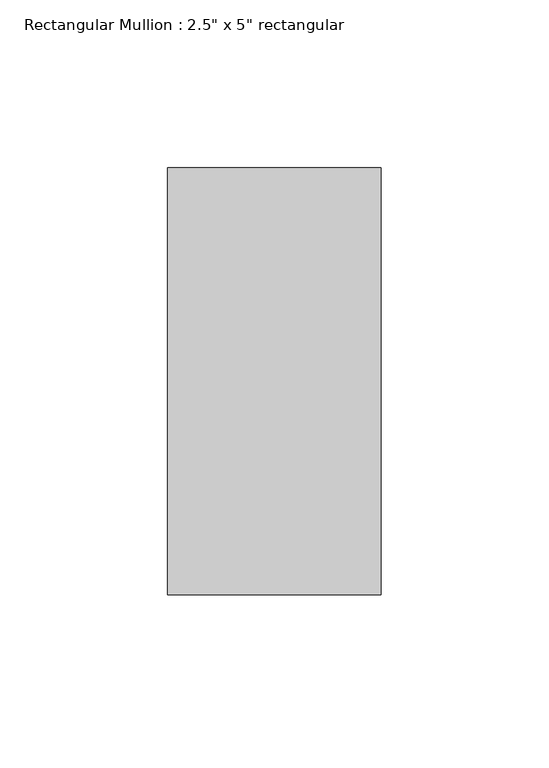
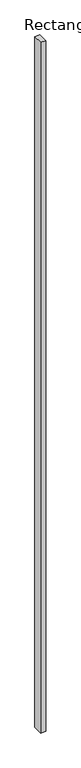
"""IFC4 building model written with IfcOpenShell, lengths in millimetres: member geometry."""

from ifc_helpers import new_model, si_unit, frame, origin, place, context, project, spatial, polyline, outline, extrude, source, transform, mapped, element, save


def member_5f6c94d3(model_context):
    return source(origin(), model_context, "Body", "SweptSolid", [
        extrude(outline(polyline([(0.0, 63.5), (0.0, -63.5), (-63.5, -63.5), (-63.5, 63.5), (0.0, 63.5)])), frame((0.0, 0.0, -9156.7), z_axis=(0.0, 0.0, 1.0), x_axis=(1.0, 0.0, 0.0)), (0.0, 0.0, 1.0), 9156.7),
    ])


if __name__ == "__main__":
    model = new_model("IFC4")
    model_context = context("Model", 3, world=origin())
    ifc_project = project(units=[si_unit("LENGTHUNIT", "METRE", prefix="MILLI")], contexts=[model_context])
    site = spatial("IfcSite", under=ifc_project)
    building = spatial("IfcBuilding", under=site)
    placement = place(None, origin())
    member_shape = member_5f6c94d3(model_context)
    element("IfcMember", 1, ObjectType="Rectangular Mullion : 2.5\" x 5\" rectangular", at=placement, inside=building, context=model_context, shape_type="MappedRepresentation", body=[
        mapped(member_shape, transform((0.0, 0.0, 0.0), x_axis=(1.0, 0.0, 0.0), y_axis=(0.0, 1.0, 0.0), z_axis=(0.0, 0.0, 1.0))),
    ])
    save(model, "model.ifc")

# Revit data of these elements
# Type "Rectangular Mullion : 2.5\" x 5\" rectangular"
#   built-in parameter 1007304 = 0.416667 (stored number, unit not read)
#   built-in parameter 1007301 = 0.104167 (stored number, unit not read)
#   built-in parameter 1007300 = 0.104167 (stored number, unit not read)
# Element 1 (IfcMember, "Rectangular Mullion : 2.5\" x 5\" rectangular")
#   Materials on its faces: "Aluminum"
# Materials
#   "Aluminum": class "Metal", colour RGB 247 247 247, transparency 0, Description = "Aluminum 6061", Cost = 0
